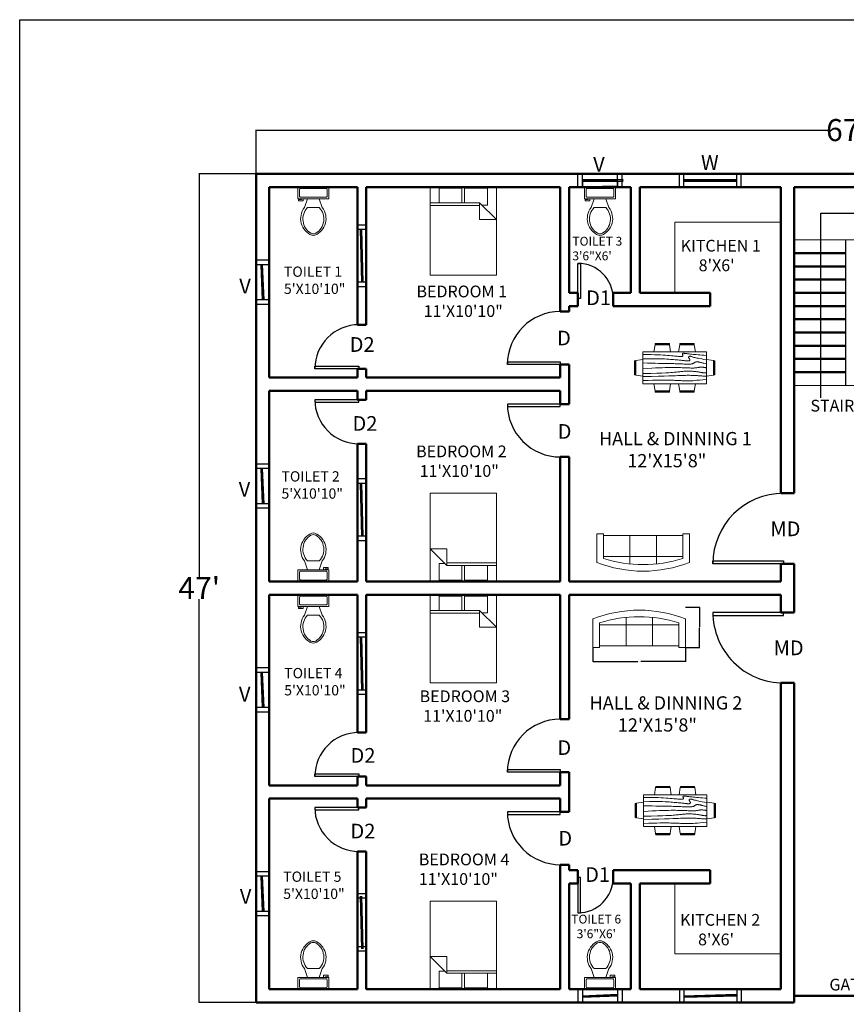
# Model space of a CAD drawing. Units: inches. Extents: x 9239 to 26065, y 6728 to 14611.
# Tile 2 of 12: x 9239 to 9801, y 7264 to 7934. Entities that reach past the tile are written whole.
import ezdxf

# ---------------------------------------------------------------- set-up
doc = ezdxf.new("R2010")
doc.units = ezdxf.units.IN
doc.header["$MEASUREMENT"] = 0
for name, color, linetype, lineweight in [('A-ANNO-DIMS', 2, 'Continuous', 18), ('A-ANNO-TEXT', 7, 'Continuous', 18), ('A-AREA-IDEN', 7, 'Continuous', 18), ('A-DOOR', 4, 'Continuous', 25), ('A-FLOR-FIXT', 8, 'Continuous', 18), ('A-FLOR-STRS', 3, 'Continuous', 25), ('A-FURN', 8, 'Continuous', 18), ('A-GLAZ', 4, 'Continuous', 25), ('A-WALL', 7, 'Continuous', 50)]:
    doc.layers.add(name, color=color, linetype=linetype, lineweight=lineweight)
doc.styles.get("Standard").update_dxf_attribs({"font": 'arial.ttf'})
doc.dimstyles.get("Standard").update_dxf_attribs({"dimtxt": 0.18, "dimasz": 0.18, "dimexe": 0.18, "dimexo": 0.0625, "dimgap": 0.09, "dimtad": 0, "dimtih": 1, "dimtoh": 1, "dimdec": 0, "dimzin": 0, "dimdsep": 46, "dimlunit": 3, "dimtxsty": 'Standard', "dimcen": 0.09, "dimadec": 0, "dimazin": 0, "dimtfac": 1, "dimtdec": 0, "dimtofl": 0, "dimtmove": 0, "dimatfit": 3, "dimfxl": 1, "dimtolj": 1, "dimtzin": 0, "dimarcsym": 0})

# ---------------------------------------------------------------- blocks, each defined once
blk = doc.blocks.new('*U6')
for p, q in [((0, 0), (0, -5)), ((24, 0), (24, -5))]:
    blk.add_line(p, q)
blk.add_lwpolyline([(0, 0), (0, 24), (1.75, 24), (1.75, 0)], close=True)
blk.add_arc((0, 0), 24, 0, 90)
blk = doc.blocks.new('*U5')
for p, q in [((0, 0), (0, 5)), ((24, 0), (24, 5))]:
    blk.add_line(p, q)
blk.add_lwpolyline([(0, 0), (0, -24), (1.75, -24), (1.75, 0)], close=True)
blk.add_arc((0, 0), 24, 270, 0)
blk = doc.blocks.new('*U8')
for p, q in [((-30, 0), (-30, 5)), ((0, 0), (0, 5))]:
    blk.add_line(p, q)
blk.add_lwpolyline([(0, 0), (0, -30), (-1.75, -30), (-1.75, 0)], close=True)
blk.add_arc((0, 0), 30, 180, 270)
blk = doc.blocks.new('*U9')
for p, q in [((0, 0), (0, 5)), ((30, 0), (30, 5))]:
    blk.add_line(p, q)
blk.add_lwpolyline([(0, 0), (0, -30), (1.75, -30), (1.75, 0)], close=True)
blk.add_arc((0, 0), 30, 270, 0)
blk = doc.blocks.new('*U14')
for p, q in [((-36, 0), (-36, 6)), ((0, 0), (0, 6))]:
    blk.add_line(p, q)
blk.add_lwpolyline([(0, 0), (0, -36), (-1.75, -36), (-1.75, 0)], close=True)
blk.add_arc((0, 0), 36, 180, 270)
blk = doc.blocks.new('*U13')
for p, q in [((0, 0), (0, 6)), ((36, 0), (36, 6))]:
    blk.add_line(p, q)
blk.add_lwpolyline([(0, 0), (0, -36), (1.75, -36), (1.75, 0)], close=True)
blk.add_arc((0, 0), 36, 270, 360)
blk = doc.blocks.new('*U12')
for p, q in [((0, 0), (0, 6)), ((40, 0), (40, 6))]:
    blk.add_line(p, q)
blk.add_lwpolyline([(0, 0), (0, -40), (1.75, -40), (1.75, 0)], close=True)
blk.add_arc((0, 0), 40, 270, 360)
blk = doc.blocks.new('*U15')
for p, q in [((-40, 0), (-40, 6)), ((0, 0), (0, 6))]:
    blk.add_line(p, q)
blk.add_lwpolyline([(0, 0), (0, -40), (-1.75, -40), (-1.75, 0)], close=True)
blk.add_arc((0, 0), 40, 180, 270)
blk = doc.blocks.new('Bed - Queen')
for p, q in [((0, -80.00003), (0, 0)), ((0, 0), (59.99999, 0)), ((59.99999, 0), (59.99999, -80.00003)), ((7.99999, -1.2), (28.79998, -1.2)), ((7.99999, -14.4), (7.99999, -1.2)), ((28.79998, -1.2), (28.79998, -14.4)), ((31.19999, -1.2), (51.99999, -1.2)), ((31.19999, -14.4), (31.19999, -1.2)), ((51.99999, -1.2), (51.99999, -16.4)), ((0, -14.4), (44.8, -14.4)), ((44.8, -16.8), (0, -16.8)), ((59.99999, -29.6), (44.8, -14.4)), ((44.8, -14.4), (44.8, -29.6)), ((51.99999, -16.4), (46.79936, -16.4)), ((44.8, -29.6), (59.99999, -29.6)), ((59.99999, -80.00003), (0, -80.00003))]:
    blk.add_line(p, q)
blk = doc.blocks.new('Toilet - top')
for p, q in [((9.5, -6), (9.5, -2)), ((-10, -8.5), (-8, -8.5)), ((-10, -9.5), (-10, -8.5)), ((-7, -9.5), (-10, -9.5)), ((-8, -8.5), (-8, -8)), ((-7, -8), (-7, -9.5)), ((-4, -8), (-6, -14)), ((4, -8), (6, -14)), ((4, -14), (-4, -14))]:
    blk.add_line(p, q)
blk.add_lwpolyline([(10.5, -8), (10.5, 0), (-10.5, 0), (-10.5, -8)], close=True)
for points in [[(-9.5, -2), (-9.5, -6)], [(8.5, -1), (-8.5, -1)], [(-8.5, -7), (8.5, -7)]]:
    blk.add_lwpolyline(points)
for centre, radius, start, end in [((-8.62, -1.88), 0.884, 81.8699, 188.1301), ((-8.62, -6.12), 0.884, 171.8699, 278.1301), ((8.62, -1.88), 0.884, 351.8699, 98.1301), ((8.62, -6.12), 0.884, 261.8699, 8.1301), ((3.52, -21.58), 12.17, 141.46911, 247.97143), ((4.2, -21.82), 11.33, 136.36773, 238.94682), ((-3.52, -21.58), 12.17, 292.02843, 38.53071), ((-4.2, -21.82), 11.33, 301.05301, 43.63209), ((0, -27.88), 4, 245.73182, 294.26817), ((0, -29), 4, 254.86053, 285.13947)]:
    blk.add_arc(centre, radius, start, end)
blk = doc.blocks.new('Sofa - Roundback 7 ft.')
for p, q in [((-12.00002, -32.4421), (-12.00003, -6.5971)), ((11.99997, -32.4421), (11.99998, -6.5971)), ((-36.000027, -34), (-36.000027, -11.4696)), ((-35.999844, -13.3819), (35.9998, -13.3819)), ((35.99998, -34), (35.99998, -11.4696)), ((-36.000027, -32.4421), (35.99998, -32.4421))]:
    blk.add_line(p, q)
for points in [[(-36.000027, -34), (-42.000027, -34), (-42.000027, -8)], [(41.99998, -8), (41.99998, -34), (35.99998, -34)]]:
    blk.add_lwpolyline(points)
for centre, radius, start, end in [((0, -114.25), 114.25, 68.43141, 111.5686), ((-0.00001, -127.1968), 121.1968, 72.72033, 107.2797)]:
    blk.add_arc(centre, radius, start, end)
blk = doc.blocks.new('Dining Set - 36 x 72 in.')
for p, q in [((-22.2343, 26.00059), (-23.4847, 17.99762)), ((-22.2304, 26), (-5.7608, 26)), ((-22, 27.5), (-22.1562, 26.50042)), ((-5.8416, 26.5), (-22.1534, 26.5)), ((-22, 27.5), (-6, 27.5)), ((-5.8437, 26.49966), (-6, 27.5)), ((-4.5152, 17.99762), (-5.7655, 25.99926)), ((5.7657, 26.00059), (4.5153, 17.99762)), ((5.7696, 26), (22.2392, 26)), ((6, 27.5), (5.8438, 26.50042)), ((22.1584, 26.5), (5.8466, 26.5)), ((6, 27.5), (22, 27.5)), ((22.1563, 26.49966), (22, 27.5)), ((23.4848, 17.99762), (22.2345, 25.99926)), ((36, 18), (-36, 18)), ((-36, 18), (-36, -18)), ((36, -18), (36, 18)), ((-45.5, 8), (-44.5004, 8.15617)), ((-45.5, 8), (-45.5, -8)), ((-44.5, -8.15843), (-44.5, 8.15338)), ((-44.0006, 8.23428), (-35.9976, 9.48474)), ((-44, 8.23041), (-44, -8.23915)), ((44.0006, 8.23428), (35.9976, 9.48474)), ((44, 8.23041), (44, -8.23915)), ((44.5, -8.15843), (44.5, 8.15338)), ((45.5, 8), (44.5005, 8.15617)), ((45.5, 8), (45.5, -8)), ((-44.4997, -8.15631), (-45.5, -8)), ((-35.9976, -9.48476), (-43.9993, -8.2345)), ((35.9976, -9.48476), (43.9993, -8.2345)), ((44.4997, -8.15631), (45.5, -8)), ((-36, -18), (36, -18)), ((-22.2343, -26.0006), (-23.4847, -17.99762)), ((-4.5152, -17.99762), (-5.7655, -25.99928)), ((5.7657, -26.0006), (4.5153, -17.99762)), ((23.4848, -17.99762), (22.2345, -25.99928)), ((-22.2304, -26), (-5.7608, -26)), ((-22, -27.5), (-22.1562, -26.50044)), ((-5.8416, -26.5), (-22.1534, -26.5)), ((-22, -27.5), (-6, -27.5)), ((-5.8437, -26.49967), (-6, -27.5)), ((5.7696, -26), (22.2392, -26)), ((6, -27.5), (5.8438, -26.50044)), ((22.1584, -26.5), (5.8466, -26.5)), ((6, -27.5), (22, -27.5)), ((22.1563, -26.49967), (22, -27.5))]:
    blk.add_line(p, q)
for points in [[(-36, 15), (-31.1772, 14.97754), (-26.8079, 14.91406), (-22.8538, 14.81543), (-19.276, 14.6875), (-16.0362, 14.53613), (-13.0957, 14.36718), (-10.4159, 14.18652), (-7.9583, 14), (-5.6904, 13.81315), (-3.6035, 13.63021), (-1.6954, 13.45508), (0.0365, 13.29166), (1.5945, 13.14388), (2.9811, 13.01562), (4.1988, 12.9108), (5.25, 12.83333), (6.1393, 12.78613), (6.8802, 12.76823), (7.4883, 12.77767), (7.9792, 12.8125), (8.3685, 12.87077), (8.6719, 12.95052), (8.9049, 13.0498), (9.0833, 13.16666), (9.2205, 13.29899), (9.3216, 13.44401), (9.3895, 13.59879), (9.4271, 13.76041), (9.4373, 13.92594), (9.4232, 14.09245), (9.3875, 14.257), (9.3333, 14.41666), (9.2638, 14.56917), (9.1836, 14.71484), (9.0975, 14.85465), (9.0104, 14.98958), (8.9272, 15.1206), (8.8529, 15.2487), (8.7922, 15.37483), (8.75, 15.5), (8.7305, 15.62467), (8.7344, 15.74739), (8.7617, 15.86621), (8.8125, 15.97916), (8.8867, 16.08431), (8.9844, 16.17968), (9.1055, 16.26334), (9.25, 16.33333), (9.4189, 16.38802), (9.6172, 16.42708), (9.8506, 16.45052), (10.125, 16.45833), (10.4463, 16.45052), (10.8203, 16.42708), (11.2529, 16.38802), (11.75, 16.33333), (12.3184, 16.26318), (12.9694, 16.17838), (13.7151, 16.07991), (14.5677, 15.96875), (15.5395, 15.84586), (16.6426, 15.71224), (17.8893, 15.56884), (19.2917, 15.41666), (20.859, 15.25667), (22.5879, 15.08984), (24.4721, 14.91715), (26.5052, 14.73958), (28.6809, 14.5581), (30.9929, 14.3737), (33.4347, 14.18733), (36, 14)], [(-36, 10), (-28.9766, 10.14274), (-23.1725, 10.20442), (-18.4241, 10.19775), (-14.5677, 10.13541), (-11.4399, 10.03011), (-8.877, 9.89453), (-6.7154, 9.74137), (-4.7917, 9.58333), (-2.9698, 9.43082), (-1.2246, 9.28515), (0.4415, 9.14534), (2.026, 9.01041), (3.5266, 8.87939), (4.9408, 8.7513), (6.266, 8.62516), (7.5, 8.5), (8.6411, 8.37549), (9.6914, 8.2539), (10.6538, 8.13818), (11.5312, 8.03125), (12.3267, 7.93603), (13.043, 7.85547), (13.6831, 7.79248), (14.25, 7.75), (14.7471, 7.7303), (15.1797, 7.73307), (15.5537, 7.75732), (15.875, 7.80208), (16.1494, 7.86637), (16.3828, 7.94922), (16.5811, 8.04964), (16.75, 8.16666), (16.8944, 8.29915), (17.0143, 8.44531), (17.1089, 8.60319), (17.1771, 8.77083), (17.218, 8.94629), (17.2305, 9.1276), (17.2137, 9.31282), (17.1667, 9.5), (17.0895, 9.6875), (16.987, 9.875), (16.8649, 10.0625), (16.7292, 10.25), (16.5856, 10.4375), (16.4401, 10.625), (16.2985, 10.8125), (16.1667, 11), (16.05, 11.18733), (15.9518, 11.3737), (15.8752, 11.5581), (15.8229, 11.73958), (15.798, 11.91715), (15.8034, 12.08984), (15.842, 12.25667), (15.9167, 12.41666), (16.0295, 12.56836), (16.1784, 12.70833), (16.3605, 12.83268), (16.5729, 12.9375), (16.8127, 13.01888), (17.0768, 13.07291), (17.3625, 13.0957), (17.6667, 13.08333), (17.9894, 13.03312), (18.3418, 12.94726), (18.7382, 12.82918), (19.1927, 12.68229), (19.7195, 12.51001), (20.3327, 12.31575), (21.0465, 12.10294), (21.875, 11.875), (22.8357, 11.63354), (23.959, 11.37304), (25.2786, 11.08618), (26.8282, 10.76562), (28.6414, 10.40405), (30.752, 9.99414), (33.1936, 9.52856), (36, 9)], [(-36, 5.5), (-30.7157, 5.3348), (-26.069, 5.20963), (-21.9946, 5.11767), (-18.4271, 5.05208), (-15.3009, 5.00602), (-12.5508, 4.97265), (-10.1112, 4.94515), (-7.9167, 4.91666), (-5.909, 4.88167), (-4.0586, 4.83984), (-2.3429, 4.79215), (-0.7396, 4.73958), (0.7739, 4.6831), (2.22, 4.6237), (3.6213, 4.56233), (5, 4.5), (6.373, 4.43782), (7.7344, 4.3776), (9.0723, 4.32129), (10.375, 4.27083), (11.6309, 4.22819), (12.8281, 4.19531), (13.9551, 4.17415), (15, 4.16666), (15.954, 4.17448), (16.819, 4.19791), (17.6001, 4.23698), (18.3021, 4.29166), (18.9299, 4.36198), (19.4883, 4.44791), (19.9823, 4.54948), (20.4167, 4.66666), (20.7969, 4.79899), (21.1302, 4.94401), (21.4245, 5.09879), (21.6875, 5.26041), (21.9271, 5.42594), (22.1511, 5.59245), (22.3672, 5.757), (22.5834, 5.91666), (22.8065, 6.06868), (23.0404, 6.21093), (23.2879, 6.34147), (23.5521, 6.45833), (23.8358, 6.55957), (24.142, 6.64323), (24.4735, 6.70735), (24.8334, 6.75), (25.2235, 6.76969), (25.642, 6.76692), (26.0858, 6.74267), (26.5521, 6.69791), (27.0379, 6.63362), (27.5404, 6.55078), (28.0565, 6.45036), (28.5834, 6.33333), (29.1242, 6.19987), (29.7071, 6.04687), (30.3661, 5.87044), (31.1354, 5.66666), (32.0493, 5.43164), (33.142, 5.16146), (34.4475, 4.85221), (36, 4.5)], [(-36, -1), (-30.7915, -0.6591), (-26.0195, -0.38216), (-21.6519, -0.16284), (-17.6563, 0.00521), (-14.0005, 0.12833), (-10.6523, 0.21289), (-7.5796, 0.26522), (-4.75, 0.29166), (-2.134, 0.29793), (0.2878, 0.28711), (2.5317, 0.26163), (4.6146, 0.22396), (6.5529, 0.17651), (8.3633, 0.12174), (10.0623, 0.06209), (11.6667, 0), (13.1899, -0.06201), (14.6341, -0.1211), (15.9982, -0.17432), (17.2813, -0.21875), (18.4823, -0.25147), (19.6003, -0.26953), (20.6343, -0.27002), (21.5834, -0.25), (22.4481, -0.20768), (23.2357, -0.14584), (23.9549, -0.06836), (24.6146, 0.02083), (25.2235, 0.11784), (25.7904, 0.21875), (26.3241, 0.31966), (26.8334, 0.41666), (27.3265, 0.50618), (27.8099, 0.58593), (28.2894, 0.65397), (28.7709, 0.70833), (29.2601, 0.74707), (29.763, 0.76823), (30.2855, 0.76985), (30.8334, 0.75), (31.4088, 0.70784), (31.9994, 0.64713), (32.589, 0.57275), (33.1615, 0.48958), (33.7008, 0.4025), (34.1908, 0.3164), (34.6153, 0.23616), (34.9584, 0.16666), (35.2099, 0.11165), (35.3848, 0.07031), (35.504, 0.04069), (35.5886, 0.02083), (35.6594, 0.00879), (35.7377, 0.0026), (35.8442, 0.00032), (36, 0)], [(-36, -6.5), (-27.1843, -6.31267), (-20.084, -6.1263), (-14.469, -5.9419), (-10.1094, -5.76042), (-6.7752, -5.58285), (-4.2363, -5.41016), (-2.2629, -5.24333), (-0.625, -5.08334), (0.8708, -4.93099), (2.2715, -4.78646), (3.5872, -4.64974), (4.8281, -4.52084), (6.0046, -4.39974), (7.127, -4.28646), (8.2053, -4.18099), (9.25, -4.08334), (10.2705, -3.99382), (11.2734, -3.91407), (12.2647, -3.84603), (13.25, -3.79167), (14.2354, -3.75293), (15.2266, -3.73177), (16.2295, -3.73015), (17.25, -3.75), (18.2912, -3.79248), (19.3451, -3.85547), (20.4009, -3.93604), (21.4479, -4.03125), (22.4754, -4.13819), (23.4727, -4.25391), (24.4289, -4.37549), (25.3334, -4.5), (26.1785, -4.62492), (26.9694, -4.74935), (27.7145, -4.87281), (28.4219, -4.99479), (29.1, -5.11483), (29.7572, -5.23242), (30.4016, -5.34709), (31.0417, -5.45834), (31.6837, -5.56437), (32.3262, -5.65821), (32.9658, -5.73153), (33.599, -5.77604), (34.2224, -5.78345), (34.8327, -5.74545), (35.4264, -5.65373), (36, -5.5)], [(-36, -10), (-26.4022, -9.81299), (-18.4675, -9.62891), (-11.9839, -9.45069), (-6.7396, -9.28125), (-2.5226, -9.12354), (0.8789, -8.98047), (3.6769, -8.85498), (6.0833, -8.75), (8.2767, -8.66765), (10.3021, -8.60677), (12.1712, -8.56543), (13.8958, -8.54167), (15.4876, -8.53353), (16.9583, -8.53907), (18.3197, -8.55632), (19.5834, -8.58334), (20.7616, -8.61841), (21.8685, -8.66081), (22.9188, -8.71004), (23.9271, -8.76563), (24.9081, -8.82707), (25.8763, -8.89388), (26.8465, -8.96558), (27.8334, -9.04167), (28.8474, -9.12118), (29.8828, -9.20117), (30.93, -9.27824), (31.9792, -9.34896), (33.0205, -9.40991), (34.0443, -9.45768), (35.0407, -9.48885), (36, -9.5)], [(-36, -14.5), (-30.0881, -14.33513), (-25.0332, -14.21224), (-20.7312, -14.12647), (-17.0781, -14.07292), (-13.97, -14.04671), (-11.3027, -14.04297), (-8.9724, -14.05681), (-6.875, -14.08334), (-4.9224, -14.11833), (-3.0905, -14.16016), (-1.3709, -14.20785), (0.2448, -14.26042), (1.7647, -14.3169), (3.1973, -14.3763), (4.5507, -14.43767), (5.8333, -14.5), (7.0554, -14.5621), (8.235, -14.62175), (9.3922, -14.67652), (10.5469, -14.72396), (11.7192, -14.76164), (12.929, -14.78711), (14.1965, -14.79794), (15.5417, -14.79167), (16.9933, -14.76424), (18.6152, -14.70508), (20.4804, -14.60197), (22.6615, -14.44271), (25.2312, -14.21509), (28.2624, -13.9069), (31.8277, -13.50594), (36, -13)]]:
    blk.add_lwpolyline(points)
blk = doc.blocks.new('*D22')
at = {"layer": 'A-ANNO-DIMS', "color": 0, "lineweight": -2, "transparency": 16777216}
for p, q in [((9399.35, 7829.13), (9399.35, 7858.98)), ((9399.53, 7858.8), (9788.49, 7858.8)), ((10203.17, 7858.8), (9814.21, 7858.8)), ((10203.35, 7829.13), (10203.35, 7858.98))]:
    blk.add_line(p, q, dxfattribs=at)
at = {"layer": 'A-ANNO-DIMS', "color": 0, "transparency": 16777216}
for points in [[(9399.53, 7858.83), (9399.53, 7858.77), (9399.35, 7858.8)], [(10203.17, 7858.83), (10203.17, 7858.77), (10203.35, 7858.8)]]:
    blk.add_solid(points, dxfattribs=at)
at = {"layer": 'Defpoints', "color": 0, "transparency": 16777216}
for p in [(10203.35, 7858.8), (9399.35, 7829.07), (10203.35, 7829.07)]:
    blk.add_point(p, dxfattribs=at)
at = {"layer": 'A-ANNO-DIMS', "color": 0, "transparency": 16777216, "insert": (9801.35, 7858.8), "char_height": 0.18, "attachment_point": 5}
blk.add_mtext("\\A1;{\\H83.33333x;67'}", dxfattribs=at)
blk = doc.blocks.new('*D23')
at = {"layer": 'A-ANNO-DIMS', "color": 0, "lineweight": -2, "transparency": 16777216}
for p, q in [((9399.29, 7829.07), (9360.53, 7829.07)), ((9360.71, 7828.89), (9360.71, 7554.66)), ((9360.71, 7265.25), (9360.71, 7539.48)), ((9399.29, 7265.07), (9360.53, 7265.07))]:
    blk.add_line(p, q, dxfattribs=at)
at = {"layer": 'A-ANNO-DIMS', "color": 0, "transparency": 16777216}
for points in [[(9360.68, 7828.89), (9360.74, 7828.89), (9360.71, 7829.07)], [(9360.68, 7265.25), (9360.74, 7265.25), (9360.71, 7265.07)]]:
    blk.add_solid(points, dxfattribs=at)
at = {"layer": 'Defpoints', "color": 0, "transparency": 16777216}
for p in [(9399.35, 7829.07), (9360.71, 7265.07), (9399.35, 7265.07)]:
    blk.add_point(p, dxfattribs=at)
at = {"layer": 'A-ANNO-DIMS', "color": 0, "transparency": 16777216, "insert": (9360.71, 7547.07), "char_height": 0.18, "attachment_point": 5}
blk.add_mtext("\\A1;{\\H83.33333x;47'}", dxfattribs=at)
blk = doc.blocks.new('WIN-36')
for p, q in [((0, 1), (36, 1)), ((0, 0.5), (36, 0.5)), ((0, 0), (36, 0))]:
    blk.add_line(p, q)
blk = doc.blocks.new('WIN-24')
for p, q in [((0, 1), (24, 1)), ((0, 0.5), (24, 0.5)), ((0, 0), (24, 0))]:
    blk.add_line(p, q)
blk = doc.blocks.new('*D42')
at = {"layer": 'A-ANNO-DIMS', "color": 0, "lineweight": -2, "transparency": 16777216}
for p, q in [((9621.35, 7824.01), (9621.35, 7820.29)), ((9645.35, 7824.01), (9645.35, 7820.29)), ((9621.53, 7820.47), (9631.64, 7820.47)), ((9645.17, 7820.47), (9635.07, 7820.47))]:
    blk.add_line(p, q, dxfattribs=at)
at = {"layer": 'A-ANNO-DIMS', "color": 0, "transparency": 16777216}
for points in [[(9621.53, 7820.5), (9621.53, 7820.44), (9621.35, 7820.47)], [(9645.17, 7820.5), (9645.17, 7820.44), (9645.35, 7820.47)]]:
    blk.add_solid(points, dxfattribs=at)
at = {"layer": 'Defpoints', "color": 0, "transparency": 16777216}
for p in [(9621.35, 7824.07), (9645.35, 7824.07), (9645.35, 7820.47)]:
    blk.add_point(p, dxfattribs=at)
at = {"layer": 'A-ANNO-DIMS', "color": 0, "transparency": 16777216, "insert": (9633.35, 7820.47), "char_height": 0.18, "attachment_point": 5}
blk.add_mtext('\\A1;WINDOW V (2\'-0") 2\'-0" TYP.', dxfattribs=at)
blk = doc.blocks.new('*D43')
at = {"layer": 'A-ANNO-DIMS', "color": 0, "lineweight": -2, "transparency": 16777216}
for p, q in [((9645.41, 7825.07), (9649.13, 7825.07)), ((9645.41, 7824.07), (9649.13, 7824.07)), ((9648.95, 7824.89), (9648.95, 7824.75)), ((9648.95, 7824.25), (9648.95, 7824.39))]:
    blk.add_line(p, q, dxfattribs=at)
at = {"layer": 'A-ANNO-DIMS', "color": 0, "transparency": 16777216}
for points in [[(9648.92, 7824.89), (9648.98, 7824.89), (9648.95, 7825.07)], [(9648.92, 7824.25), (9648.98, 7824.25), (9648.95, 7824.07)]]:
    blk.add_solid(points, dxfattribs=at)
at = {"layer": 'Defpoints', "color": 0, "transparency": 16777216}
for p in [(9645.35, 7825.07), (9645.35, 7824.07), (9648.95, 7825.07)]:
    blk.add_point(p, dxfattribs=at)
at = {"layer": 'A-ANNO-DIMS', "color": 0, "transparency": 16777216, "insert": (9648.95, 7824.57), "char_height": 0.18, "attachment_point": 5}
blk.add_mtext('\\A1;0\'-1" TYP.', dxfattribs=at)
blk = doc.blocks.new('*D52')
at = {"layer": 'A-ANNO-DIMS', "color": 0, "lineweight": -2, "transparency": 16777216}
for p, q in [((9628.56, 7506.49), (9628.56, 7496.93)), ((9691.56, 7506.49), (9691.56, 7496.93)), ((9628.74, 7497.11), (9659.05, 7497.11)), ((9691.38, 7497.11), (9661.08, 7497.11))]:
    blk.add_line(p, q, dxfattribs=at)
at = {"layer": 'A-ANNO-DIMS', "color": 0, "transparency": 16777216}
for points in [[(9628.74, 7497.14), (9628.74, 7497.08), (9628.56, 7497.11)], [(9691.38, 7497.14), (9691.38, 7497.08), (9691.56, 7497.11)]]:
    blk.add_solid(points, dxfattribs=at)
at = {"layer": 'Defpoints', "color": 0, "transparency": 16777216}
for p in [(9628.56, 7506.56), (9691.56, 7506.56), (9691.56, 7497.11)]:
    blk.add_point(p, dxfattribs=at)
at = {"layer": 'A-ANNO-DIMS', "color": 0, "transparency": 16777216, "insert": (9660.06, 7497.11), "char_height": 0.18, "attachment_point": 5}
blk.add_mtext('\\A1;SOFA 5\'-3" TYP.', dxfattribs=at)
blk = doc.blocks.new('*D53')
at = {"layer": 'A-ANNO-DIMS', "color": 0, "lineweight": -2, "transparency": 16777216}
for p, q in [((9691.63, 7534.06), (9701.19, 7534.06)), ((9701.01, 7533.88), (9701.01, 7520.49)), ((9701.01, 7506.74), (9701.01, 7520.12)), ((9691.63, 7506.56), (9701.19, 7506.56))]:
    blk.add_line(p, q, dxfattribs=at)
at = {"layer": 'A-ANNO-DIMS', "color": 0, "transparency": 16777216}
for points in [[(9700.98, 7533.88), (9701.04, 7533.88), (9701.01, 7534.06)], [(9700.98, 7506.74), (9701.04, 7506.74), (9701.01, 7506.56)]]:
    blk.add_solid(points, dxfattribs=at)
at = {"layer": 'Defpoints', "color": 0, "transparency": 16777216}
for p in [(9691.56, 7534.06), (9701.01, 7534.06), (9691.56, 7506.56)]:
    blk.add_point(p, dxfattribs=at)
at = {"layer": 'A-ANNO-DIMS', "color": 0, "transparency": 16777216, "insert": (9701.01, 7520.31), "char_height": 0.18, "attachment_point": 5}
blk.add_mtext('\\A1;2\'-3 1/2" TYP.', dxfattribs=at)

msp = doc.modelspace()

# ---------------------------------------------------------------- linework, layer by layer
at = {"layer": 'A-FLOR-FIXT'}
for p, q in [((9684.35, 7796.07), (9756.35, 7796.07)), ((9684.35, 7748.07), (9684.35, 7796.07)), ((9765.35, 7784.07), (9837.35, 7784.07)), ((9765.35, 7685.07), (9837.35, 7685.07)), ((9684.35, 7298.07), (9684.35, 7346.07)), ((9756.35, 7298.07), (9684.35, 7298.07))]:
    msp.add_line(p, q, dxfattribs=at)
at = {"layer": 'A-FLOR-STRS'}
for p, q in [((9783.59, 7676.65), (9783.59, 7802.23)), ((9783.59, 7802.23), (9820.58, 7802.23)), ((9800.35, 7784.07), (9800.35, 7685.07))]:
    msp.add_line(p, q, dxfattribs=at)
msp.add_lwpolyline([(9238.6, 7933.95), (11208.24, 7933.95), (11208.24, 6728.19), (9238.6, 6728.19)], close=True, dxfattribs=at)
at = {"layer": 'A-GLAZ'}
for p, q in [((9618.35, 7820.07), (9618.35, 7829.07)), ((9621.35, 7820.07), (9621.35, 7829.07)), ((9645.35, 7820.07), (9645.35, 7829.07)), ((9648.35, 7820.07), (9648.35, 7829.07)), ((9687.35, 7820.07), (9687.35, 7829.07)), ((9690.35, 7820.07), (9690.35, 7829.07)), ((9726.35, 7820.07), (9726.35, 7829.07)), ((9729.35, 7820.07), (9729.35, 7829.07)), ((9474.35, 7794.2), (9468.35, 7794.2)), ((9474.35, 7791.2), (9468.35, 7791.2)), ((9408.35, 7770.2), (9399.35, 7770.2)), ((9408.35, 7767.2), (9399.35, 7767.2)), ((9474.35, 7755.2), (9468.35, 7755.2)), ((9474.35, 7752.2), (9468.35, 7752.2)), ((9408.35, 7743.2), (9399.35, 7743.2)), ((9408.35, 7740.2), (9399.35, 7740.2)), ((9408.35, 7631.45), (9399.35, 7631.45)), ((9408.35, 7628.45), (9399.35, 7628.45)), ((9474.35, 7621.34), (9468.35, 7621.34)), ((9474.35, 7618.34), (9468.35, 7618.34)), ((9408.35, 7604.45), (9399.35, 7604.45)), ((9408.35, 7601.45), (9399.35, 7601.45)), ((9474.35, 7582.34), (9468.35, 7582.34)), ((9474.35, 7579.34), (9468.35, 7579.34)), ((9474.35, 7516.7), (9468.35, 7516.7)), ((9474.35, 7513.7), (9468.35, 7513.7)), ((9408.35, 7492.7), (9399.35, 7492.7)), ((9408.35, 7489.7), (9399.35, 7489.7)), ((9474.35, 7477.7), (9468.35, 7477.7)), ((9474.35, 7474.7), (9468.35, 7474.7)), ((9408.35, 7465.7), (9399.35, 7465.7)), ((9408.35, 7462.7), (9399.35, 7462.7)), ((9408.35, 7353.95), (9399.35, 7353.95)), ((9408.35, 7350.95), (9399.35, 7350.95)), ((9474.35, 7338.95), (9468.35, 7338.95)), ((9474.35, 7335.95), (9468.35, 7335.95)), ((9408.35, 7326.95), (9399.35, 7326.95)), ((9408.35, 7323.95), (9399.35, 7323.95)), ((9474.35, 7302.95), (9468.35, 7302.95)), ((9474.35, 7299.95), (9468.35, 7299.95)), ((9618.35, 7274.07), (9618.35, 7265.07)), ((9621.35, 7274.07), (9621.35, 7265.07)), ((9645.35, 7274.07), (9645.35, 7265.07)), ((9648.35, 7274.07), (9648.35, 7265.07)), ((9687.35, 7274.07), (9687.35, 7265.07)), ((9690.35, 7274.07), (9690.35, 7265.07)), ((9726.35, 7274.07), (9726.35, 7265.07)), ((9729.35, 7274.07), (9729.35, 7265.07))]:
    msp.add_line(p, q, dxfattribs=at)
at = {"layer": 'A-WALL'}
for p, q in [((9399.35, 7829.07), (10203.35, 7829.07)), ((9399.35, 7265.07), (9399.35, 7829.07)), ((9408.35, 7820.07), (9468.35, 7820.07)), ((9408.35, 7690.32), (9408.35, 7820.07)), ((9468.35, 7726.32), (9468.35, 7820.07)), ((9474.35, 7726.32), (9474.35, 7820.07)), ((9474.35, 7820.07), (9606.35, 7820.07)), ((9606.35, 7735.32), (9606.35, 7820.07)), ((9612.35, 7748.07), (9612.35, 7820.07)), ((9612.35, 7820.07), (9654.35, 7820.07)), ((9654.35, 7748.07), (9654.35, 7820.07)), ((9660.35, 7748.07), (9660.35, 7820.07)), ((9660.35, 7820.07), (9756.35, 7820.07)), ((9756.35, 7611.57), (9756.35, 7820.07)), ((9765.35, 7611.57), (9765.35, 7820.07)), ((9765.35, 7820.07), (9837.35, 7820.07)), ((9765.35, 7775.07), (9800.35, 7775.07)), ((9765.35, 7766.07), (9800.35, 7766.07)), ((9765.35, 7757.07), (9800.35, 7757.07)), ((9612.35, 7748.07), (9618.35, 7748.07)), ((9618.35, 7739.07), (9618.35, 7748.07)), ((9642.35, 7739.07), (9642.35, 7748.07)), ((9642.35, 7748.07), (9654.35, 7748.07)), ((9660.35, 7748.07), (9708.35, 7748.07)), ((9708.35, 7739.07), (9708.35, 7748.07)), ((9765.35, 7748.07), (9800.35, 7748.07)), ((9606.35, 7735.32), (9612.35, 7735.32)), ((9612.35, 7739.07), (9618.35, 7739.07)), ((9612.35, 7735.32), (9612.35, 7739.07)), ((9642.35, 7739.07), (9708.35, 7739.07)), ((9765.35, 7739.07), (9800.35, 7739.07)), ((9765.35, 7730.07), (9800.35, 7730.07)), ((9468.35, 7726.32), (9474.35, 7726.32)), ((9765.35, 7721.07), (9800.35, 7721.07)), ((9765.35, 7712.07), (9800.35, 7712.07)), ((9765.35, 7703.07), (9800.35, 7703.07)), ((9468.35, 7696.32), (9474.35, 7696.32)), ((9468.35, 7690.32), (9468.35, 7696.32)), ((9474.35, 7690.32), (9474.35, 7696.32)), ((9606.35, 7699.32), (9612.35, 7699.32)), ((9606.35, 7690.32), (9606.35, 7699.32)), ((9612.35, 7672.32), (9612.35, 7699.32)), ((9765.35, 7694.07), (9800.35, 7694.07)), ((9408.35, 7690.32), (9468.35, 7690.32)), ((9474.35, 7690.32), (9606.35, 7690.32)), ((9408.35, 7551.57), (9408.35, 7681.32)), ((9408.35, 7681.32), (9468.35, 7681.32)), ((9468.35, 7675.32), (9468.35, 7681.32)), ((9474.35, 7675.32), (9474.35, 7681.32)), ((9474.35, 7681.32), (9606.35, 7681.32)), ((9606.35, 7672.32), (9606.35, 7681.32)), ((9468.35, 7675.32), (9474.35, 7675.32)), ((9606.35, 7672.32), (9612.35, 7672.32)), ((9468.35, 7551.57), (9468.35, 7645.32)), ((9468.35, 7645.32), (9474.35, 7645.32)), ((9474.35, 7551.57), (9474.35, 7645.32)), ((9606.35, 7636.32), (9612.35, 7636.32)), ((9606.35, 7551.57), (9606.35, 7636.32)), ((9612.35, 7551.57), (9612.35, 7636.32)), ((9756.35, 7611.57), (9765.35, 7611.57)), ((9756.35, 7563.57), (9765.35, 7563.57)), ((9756.35, 7551.57), (9756.35, 7563.57)), ((9765.35, 7530.57), (9765.35, 7563.57)), ((9408.35, 7551.57), (9468.35, 7551.57)), ((9474.35, 7551.57), (9606.35, 7551.57)), ((9612.35, 7551.57), (9756.35, 7551.57)), ((9408.35, 7542.57), (9468.35, 7542.57)), ((9408.35, 7412.82), (9408.35, 7542.57)), ((9468.35, 7448.82), (9468.35, 7542.57)), ((9474.35, 7448.82), (9474.35, 7542.57)), ((9474.35, 7542.57), (9606.35, 7542.57)), ((9606.35, 7457.82), (9606.35, 7542.57)), ((9612.35, 7457.82), (9612.35, 7542.57)), ((9612.35, 7542.57), (9756.35, 7542.57)), ((9756.35, 7530.57), (9756.35, 7542.57)), ((9756.35, 7530.57), (9765.35, 7530.57)), ((9756.35, 7482.57), (9765.35, 7482.57)), ((9756.35, 7346.07), (9756.35, 7482.57)), ((9765.35, 7265.07), (9765.35, 7482.57)), ((9606.35, 7457.82), (9612.35, 7457.82)), ((9468.35, 7448.82), (9474.35, 7448.82)), ((9468.35, 7418.82), (9474.35, 7418.82)), ((9468.35, 7412.82), (9468.35, 7418.82)), ((9474.35, 7412.82), (9474.35, 7418.82)), ((9606.35, 7421.82), (9612.35, 7421.82)), ((9606.35, 7412.82), (9606.35, 7421.82)), ((9612.35, 7394.82), (9612.35, 7421.82)), ((9408.35, 7412.82), (9468.35, 7412.82)), ((9474.35, 7412.82), (9606.35, 7412.82)), ((9408.35, 7274.07), (9408.35, 7403.82)), ((9408.35, 7403.82), (9468.35, 7403.82)), ((9468.35, 7397.82), (9468.35, 7403.82)), ((9474.35, 7397.82), (9474.35, 7403.82)), ((9474.35, 7403.82), (9606.35, 7403.82)), ((9606.35, 7394.82), (9606.35, 7403.82)), ((9468.35, 7397.82), (9474.35, 7397.82)), ((9606.35, 7394.82), (9612.35, 7394.82)), ((9468.35, 7274.07), (9468.35, 7367.82)), ((9468.35, 7367.82), (9474.35, 7367.82)), ((9474.35, 7274.07), (9474.35, 7367.82)), ((9606.35, 7274.07), (9606.35, 7358.82)), ((9606.35, 7358.82), (9612.35, 7358.82)), ((9612.35, 7355.07), (9612.35, 7358.82)), ((9618.35, 7355.07), (9612.35, 7355.07)), ((9618.35, 7346.07), (9618.35, 7355.07)), ((9708.35, 7355.07), (9642.35, 7355.07)), ((9642.35, 7346.07), (9642.35, 7355.07)), ((9708.35, 7346.07), (9708.35, 7355.07)), ((9612.35, 7274.07), (9612.35, 7346.07)), ((9618.35, 7346.07), (9612.35, 7346.07)), ((9654.35, 7346.07), (9642.35, 7346.07)), ((9654.35, 7274.07), (9654.35, 7346.07)), ((9660.35, 7274.07), (9660.35, 7346.07)), ((9708.35, 7346.07), (9660.35, 7346.07)), ((9756.35, 7274.07), (9756.35, 7346.07)), ((9468.35, 7274.07), (9408.35, 7274.07)), ((9606.35, 7274.07), (9474.35, 7274.07)), ((9654.35, 7274.07), (9612.35, 7274.07)), ((9756.35, 7274.07), (9660.35, 7274.07)), ((9765.35, 7265.07), (9399.35, 7265.07)), ((9765.35, 7269.57), (9837.35, 7269.57))]:
    msp.add_line(p, q, dxfattribs=at)

# ---------------------------------------------------------------- block references
at = {"layer": 'A-DOOR'}
for name, p in [('*U6', (9618.35, 7744.07)), ('*U5', (9618.35, 7350.07))]:
    msp.add_blockref(name, p, dxfattribs=at)
at = {"layer": 'A-DOOR', "rotation": 270}
for name, p in [('*U14', (9606.35, 7699.32)), ('*U8', (9469.35, 7696.32)), ('*U9', (9469.35, 7675.32)), ('*U13', (9606.35, 7672.32)), ('*U14', (9606.35, 7421.82)), ('*U8', (9469.35, 7418.82)), ('*U9', (9469.35, 7397.82)), ('*U13', (9606.35, 7394.82))]:
    msp.add_blockref(name, p, dxfattribs=at)
for name, p, xscale, yscale, zscale in [('*U15', (9758.15, 7563.57), 1.199999999999999, 1.199999999999999, 1.199999999999999), ('*U12', (9758.15, 7530.57), 1.199999999999972, 1.199999999999972, 1.199999999999972)]:
    msp.add_blockref(name, p, dxfattribs=dict(at, xscale=xscale, yscale=yscale, zscale=zscale))
at = {"layer": 'A-FLOR-FIXT'}
for p in [(9438.35, 7820.07), (9633.35, 7820.07), (9438.35, 7542.57)]:
    msp.add_blockref('Toilet - top', p, dxfattribs=at)
at = {"layer": 'A-FLOR-FIXT', "rotation": 180}
for p in [(9438.35, 7551.57), (9438.35, 7274.07), (9633.35, 7274.07)]:
    msp.add_blockref('Toilet - top', p, dxfattribs=at)
at = {"layer": 'A-FURN'}
for name, p, xscale, yscale, zscale in [('Bed - Queen', (9517.85, 7820.07), 0.75, 0.75, 0.75), ('Dining Set - 36 x 72 in.', (9684.14, 7697.01), 0.6, 0.6, 0.6), ('Bed - Queen', (9517.85, 7542.57), 0.75, 0.75, 0.75), ('Sofa - Roundback 7 ft.', (9660.06, 7532.06), 0.75, 0.75, 0.75), ('Dining Set - 36 x 72 in.', (9684.52, 7395.64), 0.6, 0.6, 0.6)]:
    msp.add_blockref(name, p, dxfattribs=dict(at, xscale=xscale, yscale=yscale, zscale=zscale))
at = {"layer": 'A-FURN', "xscale": 0.75, "yscale": 0.75, "zscale": 0.75, "rotation": 180}
for name, p in [('Bed - Queen', (9562.85, 7551.57)), ('Sofa - Roundback 7 ft.', (9662.71, 7558.57)), ('Bed - Queen', (9562.85, 7274.07))]:
    msp.add_blockref(name, p, dxfattribs=at)
at = {"layer": 'A-GLAZ'}
for name, p in [('WIN-24', (9621.35, 7824.07)), ('WIN-36', (9690.35, 7824.07))]:
    msp.add_blockref(name, p, dxfattribs=at)
for name, p, rotation in [('WIN-36', (9472.35, 7755.22), 91.59114027121196), ('WIN-24', (9404.85, 7743.23), 92.38594403041485), ('WIN-24', (9404.85, 7604.48), 92.38594403041485), ('WIN-36', (9472.35, 7582.36), 91.59114027120035), ('WIN-36', (9472.35, 7477.72), 91.59114027120035), ('WIN-24', (9404.85, 7465.73), 92.38594403041485), ('WIN-24', (9404.85, 7326.98), 92.38594403041485), ('WIN-36', (9472.35, 7301.47), 91.59114027120035), ('WIN-24', (9621.38, 7268.57), 2.385944030397281), ('WIN-36', (9690.37, 7268.57), 1.591140271200308)]:
    msp.add_blockref(name, p, dxfattribs=dict(at, rotation=rotation))

# ---------------------------------------------------------------- texts
at = {"layer": 'A-ANNO-TEXT', "char_height": 10, "attachment_point": 1}
for s, insert in [('W', (9702.08, 7841.75)), ('V', (9628.72, 7840.56)), ('V', (9387.97, 7757.59)), ('D1', (9623.92, 7749.65)), ('D', (9604.15, 7722.28)), ('D2', (9463.07, 7717.87)), ('D2', (9464.98, 7664.12)), ('D', (9604.58, 7658.68)), ('V', (9387.58, 7619.37)), ('MD', (9749.26, 7592.41)), ('MD', (9751.44, 7511.41)), ('V', (9387.74, 7479.87)), ('D', (9604.39, 7443.47)), ('D2', (9463.64, 7438.19)), ('D2', (9463.61, 7386.68)), ('D', (9605.01, 7381.79)), ('D1', (9623.26, 7357.09)), ('V', (9388.35, 7342.28))]:
    msp.add_mtext_dynamic_manual_height_columns(s, width=325.9721, gutter_width=1, heights=[0], dxfattribs=dict(at, insert=insert))
at = {"layer": 'A-AREA-IDEN', "attachment_point": 1}
for s, width, insert, char_height in [('TOILET 3\\P3\'6"X6\'', 628.3357, (9614.58, 7786.17), 6), ("KITCHEN 1\\P     8'X6'", 630.614, (9688.27, 7784.11), 8), ('TOILET 1\\P5\'X10\'10"', 821.2141, (9418.35, 7765.94), 7), ('BEDROOM 1\\P  11\'X10\'10"', 955.6877, (9508.52, 7752.97), 8), ('STAIRE', 401.4252, (9776.53, 7675.22), 8), ('HALL & DINNING 1\\P       12\'X15\'8"', 841.4884, (9632.69, 7653.31), 9), ('BEDROOM 2\\P 11\'X10\'10"', 775.7152, (9508.26, 7644.12), 8), ('TOILET 2\\P5\'X10\'10"', 719.9641, (9416.69, 7626.6), 7), ('TOILET 4\\P5\'X10\'10"', 448.8027, (9418.55, 7492.7), 7), ('BEDROOM 3\\P 11\'X10\'10"', 964.9294, (9510.63, 7477.44), 8), ('HALL & DINNING 2\\P       12\'X15\'8"', 905.9693, (9626.29, 7473.43), 9), ('BEDROOM 4\\P11\'X10\'10"', 433.9289, (9510.1, 7366.38), 8), ('TOILET 5\\P5\'X10\'10"', 1635.8082, (9417.87, 7354.15), 7), ("KITCHEN 2\\P     8'X6'", 915.899, (9687.86, 7325.26), 8), ('TOILET 6\\P  3\'6"X6\'', 190.7057, (9613.81, 7324.76), 6), ('GATE', 401.4252, (9789.43, 7281.18), 8)]:
    msp.add_mtext_dynamic_manual_height_columns(s, width=width, gutter_width=1, heights=[0], dxfattribs=dict(at, insert=insert, char_height=char_height))

# ---------------------------------------------------------------- dimensions: what is measured, and where the dimension line sits
at = {"layer": 'A-ANNO-DIMS'}
dim = msp.add_linear_dim(base=(10203.35, 7858.8), p1=(9399.35, 7829.07), p2=(10203.35, 7829.07), text='{\\H83.33333x;<>}', dimstyle='Standard', override={"dimclrd": 0, "dimclre": 0, "dimclrt": 0}, dxfattribs=at)
dim.commit()
dim.dimension.update_dxf_attribs({"geometry": '*D22', "text_midpoint": (9801.35, 7858.8), "dimtype": 160})
dim = msp.add_linear_dim(base=(9360.71, 7265.07), p1=(9399.35, 7829.07), p2=(9399.35, 7265.07), angle=90, text='{\\H83.33333x;<>}', dimstyle='Standard', override={"dimclrd": 0, "dimclre": 0, "dimclrt": 0}, dxfattribs=at)
dim.commit()
dim.dimension.update_dxf_attribs({"geometry": '*D23', "text_midpoint": (9360.71, 7547.07), "dimtype": 160})
for base, p1, p2, text, picture, middle in [((9645.35, 7820.47), (9621.35, 7824.07), (9645.35, 7824.07), 'WINDOW V (2\'-0") <> TYP.', '*D42', (9633.35, 7820.47)), ((9691.56, 7497.11), (9628.56, 7506.56), (9691.56, 7506.56), 'SOFA <> TYP.', '*D52', (9660.06, 7497.11))]:
    dim = msp.add_linear_dim(base=base, p1=p1, p2=p2, text=text, dimstyle='Standard', override={"dimdec": 1, "dimlfac": 1, "dimrnd": 0, "dimzin": 1, "dimdsep": 46, "dimlunit": 4, "dimfrac": 2}, dxfattribs=at)
    dim.commit()
    dim.dimension.update_dxf_attribs({"geometry": picture, "text_midpoint": middle})
for base, p1, p2, picture, middle in [((9648.95, 7825.07), (9645.35, 7824.07), (9645.35, 7825.07), '*D43', (9648.95, 7824.57)), ((9701.01, 7534.06), (9691.56, 7506.56), (9691.56, 7534.06), '*D53', (9701.01, 7520.31))]:
    dim = msp.add_linear_dim(base=base, p1=p1, p2=p2, angle=90, text='<> TYP.', dimstyle='Standard', override={"dimdec": 1, "dimlfac": 1, "dimrnd": 0, "dimzin": 1, "dimdsep": 46, "dimlunit": 4, "dimfrac": 2}, dxfattribs=at)
    dim.commit()
    dim.dimension.update_dxf_attribs({"geometry": picture, "text_midpoint": middle})

doc.saveas('drawing.dxf')
